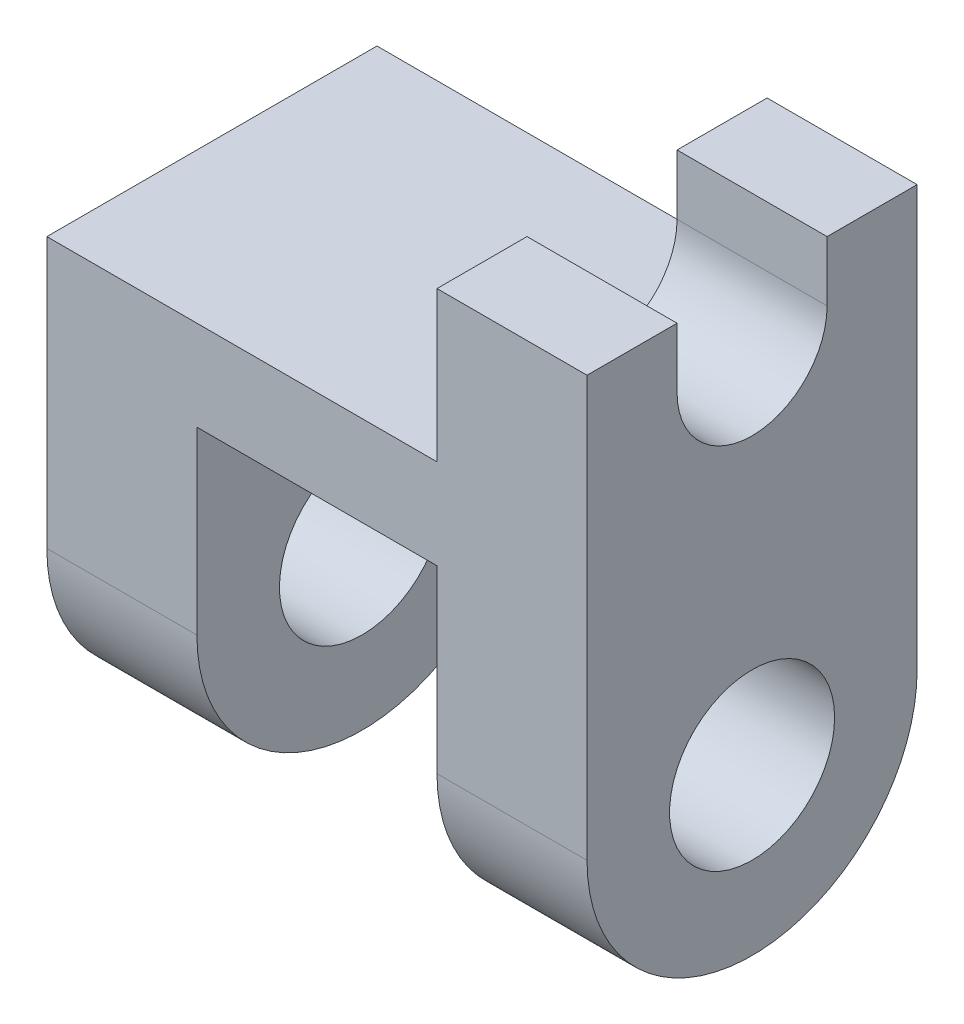
ISO-10303-21;
HEADER;
FILE_DESCRIPTION(('STEP AP214'),'2;1');
FILE_NAME('part.step','',(''),(''),'','','');
FILE_SCHEMA(('AUTOMOTIVE_DESIGN { 1 0 10303 214 1 1 1 1 }'));
ENDSEC;
DATA;
#1=APPLICATION_CONTEXT('core data for automotive mechanical design processes');
#2=APPLICATION_PROTOCOL_DEFINITION('international standard','automotive_design',2000,#1);
#3=PRODUCT_CONTEXT('',#1,'mechanical');
#4=PRODUCT('Part','Part','',(#3));
#5=PRODUCT_RELATED_PRODUCT_CATEGORY('part','',(#4));
#6=PRODUCT_DEFINITION_FORMATION('','',#4);
#7=PRODUCT_DEFINITION_CONTEXT('part definition',#1,'design');
#8=PRODUCT_DEFINITION('design','',#6,#7);
#9=PRODUCT_DEFINITION_SHAPE('','',#8);
#10=(LENGTH_UNIT() NAMED_UNIT(*) SI_UNIT(.MILLI.,.METRE.));
#11=(NAMED_UNIT(*) PLANE_ANGLE_UNIT() SI_UNIT($,.RADIAN.));
#12=(NAMED_UNIT(*) SI_UNIT($,.STERADIAN.) SOLID_ANGLE_UNIT());
#13=UNCERTAINTY_MEASURE_WITH_UNIT(LENGTH_MEASURE(1.E-05),#10,'distance_accuracy_value','');
#14=(GEOMETRIC_REPRESENTATION_CONTEXT(3) GLOBAL_UNCERTAINTY_ASSIGNED_CONTEXT((#13)) GLOBAL_UNIT_ASSIGNED_CONTEXT((#10,
#11,#12)) REPRESENTATION_CONTEXT('',''));
#15=CARTESIAN_POINT('',(0.,0.,0.));
#16=DIRECTION('',(0.,0.,1.));
#17=DIRECTION('',(1.,0.,0.));
#18=AXIS2_PLACEMENT_3D('',#15,#16,#17);
#19=CARTESIAN_POINT('',(36.,32.,22.));
#20=DIRECTION('',(0.,-1.,0.));
#21=DIRECTION('',(0.,0.,-1.));
#22=AXIS2_PLACEMENT_3D('',#19,#20,#21);
#23=PLANE('',#22);
#24=DIRECTION('',(1.,0.,0.));
#25=VECTOR('',#24,1.);
#26=CARTESIAN_POINT('',(-167.635824222232,32.,10.));
#27=LINE('',#26,#25);
#28=CARTESIAN_POINT('',(16.,32.,10.));
#29=VERTEX_POINT('',#28);
#30=CARTESIAN_POINT('',(36.,32.,10.));
#31=VERTEX_POINT('',#30);
#32=EDGE_CURVE('E161',#29,#31,#27,.T.);
#33=ORIENTED_EDGE('',*,*,#32,.F.);
#34=DIRECTION('',(0.,0.,-1.));
#35=VECTOR('',#34,1.);
#36=CARTESIAN_POINT('',(16.,32.,22.));
#37=LINE('',#36,#35);
#38=CARTESIAN_POINT('',(16.,32.,22.));
#39=VERTEX_POINT('',#38);
#40=EDGE_CURVE('E147',#39,#29,#37,.T.);
#41=ORIENTED_EDGE('',*,*,#40,.F.);
#42=DIRECTION('',(-1.,0.,0.));
#43=VECTOR('',#42,1.);
#44=CARTESIAN_POINT('',(36.,32.,22.));
#45=LINE('',#44,#43);
#46=CARTESIAN_POINT('',(36.,32.,22.));
#47=VERTEX_POINT('',#46);
#48=EDGE_CURVE('E224',#47,#39,#45,.T.);
#49=ORIENTED_EDGE('',*,*,#48,.F.);
#50=DIRECTION('',(0.,0.,-1.));
#51=VECTOR('',#50,1.);
#52=CARTESIAN_POINT('',(36.,32.,22.));
#53=LINE('',#52,#51);
#54=EDGE_CURVE('E11',#47,#31,#53,.T.);
#55=ORIENTED_EDGE('',*,*,#54,.T.);
#56=EDGE_LOOP('',(#33,#41,#49,#55));
#57=FACE_BOUND('',#56,.T.);
#58=ADVANCED_FACE('F39',(#57),#23,.F.);
#59=CARTESIAN_POINT('',(16.,32.,22.));
#60=DIRECTION('',(1.,0.,0.));
#61=DIRECTION('',(0.,0.,-1.));
#62=AXIS2_PLACEMENT_3D('',#59,#60,#61);
#63=PLANE('',#62);
#64=ORIENTED_EDGE('',*,*,#40,.T.);
#65=DIRECTION('',(0.,-1.,0.));
#66=VECTOR('',#65,1.);
#67=CARTESIAN_POINT('',(16.,24.,10.));
#68=LINE('',#67,#66);
#69=CARTESIAN_POINT('',(16.,24.,10.));
#70=VERTEX_POINT('',#69);
#71=EDGE_CURVE('E140',#29,#70,#68,.T.);
#72=ORIENTED_EDGE('',*,*,#71,.T.);
#73=CARTESIAN_POINT('',(16.,24.,0.));
#74=DIRECTION('',(1.,0.,0.));
#75=DIRECTION('',(0.,0.,-1.));
#76=AXIS2_PLACEMENT_3D('',#73,#74,#75);
#77=CIRCLE('',#76,10.);
#78=CARTESIAN_POINT('',(16.,24.,-10.));
#79=VERTEX_POINT('',#78);
#80=EDGE_CURVE('E145',#70,#79,#77,.T.);
#81=ORIENTED_EDGE('',*,*,#80,.T.);
#82=DIRECTION('',(0.,1.,0.));
#83=VECTOR('',#82,1.);
#84=CARTESIAN_POINT('',(16.,24.,-10.));
#85=LINE('',#84,#83);
#86=CARTESIAN_POINT('',(16.,32.,-10.));
#87=VERTEX_POINT('',#86);
#88=EDGE_CURVE('E157',#79,#87,#85,.T.);
#89=ORIENTED_EDGE('',*,*,#88,.T.);
#90=CARTESIAN_POINT('',(16.,32.,-22.));
#91=VERTEX_POINT('',#90);
#92=EDGE_CURVE('E252',#87,#91,#37,.T.);
#93=ORIENTED_EDGE('',*,*,#92,.T.);
#94=DIRECTION('',(0.,-1.,0.));
#95=VECTOR('',#94,1.);
#96=CARTESIAN_POINT('',(16.,32.,-22.));
#97=LINE('',#96,#95);
#98=CARTESIAN_POINT('',(16.,12.,-22.));
#99=VERTEX_POINT('',#98);
#100=EDGE_CURVE('E239',#91,#99,#97,.T.);
#101=ORIENTED_EDGE('',*,*,#100,.T.);
#102=DIRECTION('',(0.,0.,-1.));
#103=VECTOR('',#102,1.);
#104=CARTESIAN_POINT('',(16.,12.,22.));
#105=LINE('',#104,#103);
#106=CARTESIAN_POINT('',(16.,12.,22.));
#107=VERTEX_POINT('',#106);
#108=EDGE_CURVE('E248',#107,#99,#105,.T.);
#109=ORIENTED_EDGE('',*,*,#108,.F.);
#110=DIRECTION('',(0.,-1.,0.));
#111=VECTOR('',#110,1.);
#112=CARTESIAN_POINT('',(16.,32.,22.));
#113=LINE('',#112,#111);
#114=EDGE_CURVE('E221',#39,#107,#113,.T.);
#115=ORIENTED_EDGE('',*,*,#114,.F.);
#116=EDGE_LOOP('',(#64,#72,#81,#89,#93,#101,#109,#115));
#117=FACE_BOUND('',#116,.T.);
#118=ADVANCED_FACE('F142',(#117),#63,.F.);
#119=CARTESIAN_POINT('',(-36.,0.,22.));
#120=DIRECTION('',(0.,1.,0.));
#121=DIRECTION('',(0.,0.,1.));
#122=AXIS2_PLACEMENT_3D('',#119,#120,#121);
#123=PLANE('',#122);
#124=DIRECTION('',(0.,0.,1.));
#125=VECTOR('',#124,1.);
#126=CARTESIAN_POINT('',(-16.,0.,22.));
#127=LINE('',#126,#125);
#128=CARTESIAN_POINT('',(-16.,0.,-22.));
#129=VERTEX_POINT('',#128);
#130=CARTESIAN_POINT('',(-16.,0.,22.));
#131=VERTEX_POINT('',#130);
#132=EDGE_CURVE('E193',#129,#131,#127,.T.);
#133=ORIENTED_EDGE('',*,*,#132,.F.);
#134=DIRECTION('',(1.,0.,0.));
#135=VECTOR('',#134,1.);
#136=CARTESIAN_POINT('',(-36.,0.,-22.));
#137=LINE('',#136,#135);
#138=CARTESIAN_POINT('',(16.,0.,-22.));
#139=VERTEX_POINT('',#138);
#140=EDGE_CURVE('E222',#129,#139,#137,.T.);
#141=ORIENTED_EDGE('',*,*,#140,.T.);
#142=DIRECTION('',(0.,0.,-1.));
#143=VECTOR('',#142,1.);
#144=CARTESIAN_POINT('',(16.,0.,22.));
#145=LINE('',#144,#143);
#146=CARTESIAN_POINT('',(16.,0.,22.));
#147=VERTEX_POINT('',#146);
#148=EDGE_CURVE('E203',#147,#139,#145,.T.);
#149=ORIENTED_EDGE('',*,*,#148,.F.);
#150=DIRECTION('',(1.,0.,0.));
#151=VECTOR('',#150,1.);
#152=CARTESIAN_POINT('',(-36.,0.,22.));
#153=LINE('',#152,#151);
#154=EDGE_CURVE('E233',#131,#147,#153,.T.);
#155=ORIENTED_EDGE('',*,*,#154,.F.);
#156=EDGE_LOOP('',(#133,#141,#149,#155));
#157=FACE_BOUND('',#156,.T.);
#158=ADVANCED_FACE('F303',(#157),#123,.F.);
#159=CARTESIAN_POINT('',(36.,0.,22.));
#160=DIRECTION('',(-1.,0.,0.));
#161=DIRECTION('',(0.,0.,1.));
#162=AXIS2_PLACEMENT_3D('',#159,#160,#161);
#163=PLANE('',#162);
#164=DIRECTION('',(0.,1.,0.));
#165=VECTOR('',#164,1.);
#166=CARTESIAN_POINT('',(36.,24.,-10.));
#167=LINE('',#166,#165);
#168=CARTESIAN_POINT('',(36.,24.,-10.));
#169=VERTEX_POINT('',#168);
#170=CARTESIAN_POINT('',(36.,32.,-10.));
#171=VERTEX_POINT('',#170);
#172=EDGE_CURVE('E53',#169,#171,#167,.T.);
#173=ORIENTED_EDGE('',*,*,#172,.F.);
#174=CARTESIAN_POINT('',(36.,24.,0.));
#175=DIRECTION('',(1.,0.,0.));
#176=DIRECTION('',(0.,0.,-1.));
#177=AXIS2_PLACEMENT_3D('',#174,#175,#176);
#178=CIRCLE('',#177,10.);
#179=CARTESIAN_POINT('',(36.,24.,10.));
#180=VERTEX_POINT('',#179);
#181=EDGE_CURVE('E59',#180,#169,#178,.T.);
#182=ORIENTED_EDGE('',*,*,#181,.F.);
#183=DIRECTION('',(0.,-1.,0.));
#184=VECTOR('',#183,1.);
#185=CARTESIAN_POINT('',(36.,24.,10.));
#186=LINE('',#185,#184);
#187=EDGE_CURVE('E163',#31,#180,#186,.T.);
#188=ORIENTED_EDGE('',*,*,#187,.F.);
#189=ORIENTED_EDGE('',*,*,#54,.F.);
#190=DIRECTION('',(0.,1.,0.));
#191=VECTOR('',#190,1.);
#192=CARTESIAN_POINT('',(36.,0.,22.));
#193=LINE('',#192,#191);
#194=CARTESIAN_POINT('',(36.,-24.,22.));
#195=VERTEX_POINT('',#194);
#196=EDGE_CURVE('E218',#195,#47,#193,.T.);
#197=ORIENTED_EDGE('',*,*,#196,.F.);
#198=CARTESIAN_POINT('',(36.,-24.,0.));
#199=DIRECTION('',(1.,0.,0.));
#200=DIRECTION('',(0.,0.,-1.));
#201=AXIS2_PLACEMENT_3D('',#198,#199,#200);
#202=CIRCLE('',#201,22.);
#203=CARTESIAN_POINT('',(36.,-24.,-22.));
#204=VERTEX_POINT('',#203);
#205=EDGE_CURVE('E175',#195,#204,#202,.T.);
#206=ORIENTED_EDGE('',*,*,#205,.T.);
#207=DIRECTION('',(0.,1.,0.));
#208=VECTOR('',#207,1.);
#209=CARTESIAN_POINT('',(36.,0.,-22.));
#210=LINE('',#209,#208);
#211=CARTESIAN_POINT('',(36.,32.,-22.));
#212=VERTEX_POINT('',#211);
#213=EDGE_CURVE('E210',#204,#212,#210,.T.);
#214=ORIENTED_EDGE('',*,*,#213,.T.);
#215=EDGE_CURVE('E50',#171,#212,#53,.T.);
#216=ORIENTED_EDGE('',*,*,#215,.F.);
#217=EDGE_LOOP('',(#173,#182,#188,#189,#197,#206,#214,#216));
#218=FACE_BOUND('',#217,.T.);
#219=CARTESIAN_POINT('',(36.,-24.,0.));
#220=DIRECTION('',(1.,0.,0.));
#221=DIRECTION('',(0.,0.,-1.));
#222=AXIS2_PLACEMENT_3D('',#219,#220,#221);
#223=CIRCLE('',#222,11.);
#224=CARTESIAN_POINT('',(36.,-24.,-11.));
#225=VERTEX_POINT('',#224);
#226=EDGE_CURVE('E162',#225,#225,#223,.T.);
#227=ORIENTED_EDGE('',*,*,#226,.F.);
#228=EDGE_LOOP('',(#227));
#229=FACE_BOUND('',#228,.T.);
#230=ADVANCED_FACE('F41',(#218,#229),#163,.F.);
#231=ORIENTED_EDGE('',*,*,#92,.F.);
#232=DIRECTION('',(1.,0.,0.));
#233=VECTOR('',#232,1.);
#234=CARTESIAN_POINT('',(-167.635824222232,32.,-10.));
#235=LINE('',#234,#233);
#236=EDGE_CURVE('E354',#87,#171,#235,.T.);
#237=ORIENTED_EDGE('',*,*,#236,.T.);
#238=ORIENTED_EDGE('',*,*,#215,.T.);
#239=DIRECTION('',(-1.,0.,0.));
#240=VECTOR('',#239,1.);
#241=CARTESIAN_POINT('',(36.,32.,-22.));
#242=LINE('',#241,#240);
#243=EDGE_CURVE('E240',#212,#91,#242,.T.);
#244=ORIENTED_EDGE('',*,*,#243,.T.);
#245=EDGE_LOOP('',(#231,#237,#238,#244));
#246=FACE_BOUND('',#245,.T.);
#247=ADVANCED_FACE('F259',(#246),#23,.F.);
#248=CARTESIAN_POINT('',(16.,12.,22.));
#249=DIRECTION('',(0.,-1.,0.));
#250=DIRECTION('',(1.,0.,0.));
#251=AXIS2_PLACEMENT_3D('',#248,#249,#250);
#252=PLANE('',#251);
#253=DIRECTION('',(-1.,0.,0.));
#254=VECTOR('',#253,1.);
#255=CARTESIAN_POINT('',(16.,12.,-22.));
#256=LINE('',#255,#254);
#257=CARTESIAN_POINT('',(-36.,12.,-22.));
#258=VERTEX_POINT('',#257);
#259=EDGE_CURVE('E245',#99,#258,#256,.T.);
#260=ORIENTED_EDGE('',*,*,#259,.T.);
#261=DIRECTION('',(0.,0.,-1.));
#262=VECTOR('',#261,1.);
#263=CARTESIAN_POINT('',(-36.,12.,22.));
#264=LINE('',#263,#262);
#265=CARTESIAN_POINT('',(-36.,12.,22.));
#266=VERTEX_POINT('',#265);
#267=EDGE_CURVE('E234',#266,#258,#264,.T.);
#268=ORIENTED_EDGE('',*,*,#267,.F.);
#269=DIRECTION('',(-1.,0.,0.));
#270=VECTOR('',#269,1.);
#271=CARTESIAN_POINT('',(16.,12.,22.));
#272=LINE('',#271,#270);
#273=EDGE_CURVE('E227',#107,#266,#272,.T.);
#274=ORIENTED_EDGE('',*,*,#273,.F.);
#275=ORIENTED_EDGE('',*,*,#108,.T.);
#276=EDGE_LOOP('',(#260,#268,#274,#275));
#277=FACE_BOUND('',#276,.T.);
#278=ADVANCED_FACE('F269',(#277),#252,.F.);
#279=CARTESIAN_POINT('',(-36.,12.,22.));
#280=DIRECTION('',(1.,0.,0.));
#281=DIRECTION('',(0.,1.,0.));
#282=AXIS2_PLACEMENT_3D('',#279,#280,#281);
#283=PLANE('',#282);
#284=DIRECTION('',(0.,-1.,0.));
#285=VECTOR('',#284,1.);
#286=CARTESIAN_POINT('',(-36.,12.,-22.));
#287=LINE('',#286,#285);
#288=CARTESIAN_POINT('',(-36.,-24.,-22.));
#289=VERTEX_POINT('',#288);
#290=EDGE_CURVE('E242',#258,#289,#287,.T.);
#291=ORIENTED_EDGE('',*,*,#290,.T.);
#292=CARTESIAN_POINT('',(-36.,-24.,0.));
#293=DIRECTION('',(-1.,0.,0.));
#294=DIRECTION('',(0.,-1.,0.));
#295=AXIS2_PLACEMENT_3D('',#292,#293,#294);
#296=CIRCLE('',#295,22.);
#297=CARTESIAN_POINT('',(-36.,-24.,22.));
#298=VERTEX_POINT('',#297);
#299=EDGE_CURVE('E185',#289,#298,#296,.T.);
#300=ORIENTED_EDGE('',*,*,#299,.T.);
#301=DIRECTION('',(0.,-1.,0.));
#302=VECTOR('',#301,1.);
#303=CARTESIAN_POINT('',(-36.,12.,22.));
#304=LINE('',#303,#302);
#305=EDGE_CURVE('E230',#266,#298,#304,.T.);
#306=ORIENTED_EDGE('',*,*,#305,.F.);
#307=ORIENTED_EDGE('',*,*,#267,.T.);
#308=EDGE_LOOP('',(#291,#300,#306,#307));
#309=FACE_BOUND('',#308,.T.);
#310=CARTESIAN_POINT('',(-36.,-24.,0.));
#311=DIRECTION('',(-1.,0.,0.));
#312=DIRECTION('',(0.,-1.,0.));
#313=AXIS2_PLACEMENT_3D('',#310,#311,#312);
#314=CIRCLE('',#313,11.);
#315=CARTESIAN_POINT('',(-36.,-35.,0.));
#316=VERTEX_POINT('',#315);
#317=EDGE_CURVE('E176',#316,#316,#314,.T.);
#318=ORIENTED_EDGE('',*,*,#317,.F.);
#319=EDGE_LOOP('',(#318));
#320=FACE_BOUND('',#319,.T.);
#321=ADVANCED_FACE('F272',(#309,#320),#283,.F.);
#322=CARTESIAN_POINT('',(0.,0.,22.));
#323=DIRECTION('',(0.,0.,1.));
#324=DIRECTION('',(1.,0.,0.));
#325=AXIS2_PLACEMENT_3D('',#322,#323,#324);
#326=PLANE('',#325);
#327=ORIENTED_EDGE('',*,*,#196,.T.);
#328=ORIENTED_EDGE('',*,*,#48,.T.);
#329=ORIENTED_EDGE('',*,*,#114,.T.);
#330=ORIENTED_EDGE('',*,*,#273,.T.);
#331=ORIENTED_EDGE('',*,*,#305,.T.);
#332=DIRECTION('',(-1.,0.,0.));
#333=VECTOR('',#332,1.);
#334=CARTESIAN_POINT('',(-36.,-24.,22.));
#335=LINE('',#334,#333);
#336=CARTESIAN_POINT('',(-16.,-24.,22.));
#337=VERTEX_POINT('',#336);
#338=EDGE_CURVE('E191',#337,#298,#335,.T.);
#339=ORIENTED_EDGE('',*,*,#338,.F.);
#340=DIRECTION('',(0.,1.,0.));
#341=VECTOR('',#340,1.);
#342=CARTESIAN_POINT('',(-16.,-24.,22.));
#343=LINE('',#342,#341);
#344=EDGE_CURVE('E197',#337,#131,#343,.T.);
#345=ORIENTED_EDGE('',*,*,#344,.T.);
#346=ORIENTED_EDGE('',*,*,#154,.T.);
#347=DIRECTION('',(0.,1.,0.));
#348=VECTOR('',#347,1.);
#349=CARTESIAN_POINT('',(16.,-24.,22.));
#350=LINE('',#349,#348);
#351=CARTESIAN_POINT('',(16.,-24.,22.));
#352=VERTEX_POINT('',#351);
#353=EDGE_CURVE('E189',#352,#147,#350,.T.);
#354=ORIENTED_EDGE('',*,*,#353,.F.);
#355=DIRECTION('',(-1.,0.,0.));
#356=VECTOR('',#355,1.);
#357=CARTESIAN_POINT('',(36.,-24.,22.));
#358=LINE('',#357,#356);
#359=EDGE_CURVE('E216',#195,#352,#358,.T.);
#360=ORIENTED_EDGE('',*,*,#359,.F.);
#361=EDGE_LOOP('',(#327,#328,#329,#330,#331,#339,#345,#346,#354,#360));
#362=FACE_BOUND('',#361,.T.);
#363=ADVANCED_FACE('F277',(#362),#326,.T.);
#364=CARTESIAN_POINT('',(0.,0.,-22.));
#365=DIRECTION('',(0.,0.,1.));
#366=DIRECTION('',(1.,0.,0.));
#367=AXIS2_PLACEMENT_3D('',#364,#365,#366);
#368=PLANE('',#367);
#369=ORIENTED_EDGE('',*,*,#213,.F.);
#370=DIRECTION('',(1.,0.,0.));
#371=VECTOR('',#370,1.);
#372=CARTESIAN_POINT('',(16.,-24.,-22.));
#373=LINE('',#372,#371);
#374=CARTESIAN_POINT('',(16.,-24.,-22.));
#375=VERTEX_POINT('',#374);
#376=EDGE_CURVE('E214',#375,#204,#373,.T.);
#377=ORIENTED_EDGE('',*,*,#376,.F.);
#378=DIRECTION('',(0.,1.,0.));
#379=VECTOR('',#378,1.);
#380=CARTESIAN_POINT('',(16.,-24.,-22.));
#381=LINE('',#380,#379);
#382=EDGE_CURVE('E208',#375,#139,#381,.T.);
#383=ORIENTED_EDGE('',*,*,#382,.T.);
#384=ORIENTED_EDGE('',*,*,#140,.F.);
#385=DIRECTION('',(0.,1.,0.));
#386=VECTOR('',#385,1.);
#387=CARTESIAN_POINT('',(-16.,-24.,-22.));
#388=LINE('',#387,#386);
#389=CARTESIAN_POINT('',(-16.,-24.,-22.));
#390=VERTEX_POINT('',#389);
#391=EDGE_CURVE('E205',#390,#129,#388,.T.);
#392=ORIENTED_EDGE('',*,*,#391,.F.);
#393=DIRECTION('',(1.,0.,0.));
#394=VECTOR('',#393,1.);
#395=CARTESIAN_POINT('',(-16.,-24.,-22.));
#396=LINE('',#395,#394);
#397=EDGE_CURVE('E192',#289,#390,#396,.T.);
#398=ORIENTED_EDGE('',*,*,#397,.F.);
#399=ORIENTED_EDGE('',*,*,#290,.F.);
#400=ORIENTED_EDGE('',*,*,#259,.F.);
#401=ORIENTED_EDGE('',*,*,#100,.F.);
#402=ORIENTED_EDGE('',*,*,#243,.F.);
#403=EDGE_LOOP('',(#369,#377,#383,#384,#392,#398,#399,#400,#401,#402));
#404=FACE_BOUND('',#403,.T.);
#405=ADVANCED_FACE('F265',(#404),#368,.F.);
#406=CARTESIAN_POINT('',(16.,-24.,22.));
#407=DIRECTION('',(1.,0.,0.));
#408=DIRECTION('',(0.,0.,-1.));
#409=AXIS2_PLACEMENT_3D('',#406,#407,#408);
#410=PLANE('',#409);
#411=ORIENTED_EDGE('',*,*,#382,.F.);
#412=CARTESIAN_POINT('',(16.,-24.,0.));
#413=DIRECTION('',(1.,0.,0.));
#414=DIRECTION('',(0.,0.,-1.));
#415=AXIS2_PLACEMENT_3D('',#412,#413,#414);
#416=CIRCLE('',#415,22.);
#417=EDGE_CURVE('E172',#352,#375,#416,.T.);
#418=ORIENTED_EDGE('',*,*,#417,.F.);
#419=ORIENTED_EDGE('',*,*,#353,.T.);
#420=ORIENTED_EDGE('',*,*,#148,.T.);
#421=EDGE_LOOP('',(#411,#418,#419,#420));
#422=FACE_BOUND('',#421,.T.);
#423=CARTESIAN_POINT('',(16.,-24.,0.));
#424=DIRECTION('',(1.,0.,0.));
#425=DIRECTION('',(0.,0.,-1.));
#426=AXIS2_PLACEMENT_3D('',#423,#424,#425);
#427=CIRCLE('',#426,11.);
#428=CARTESIAN_POINT('',(16.,-24.,-11.));
#429=VERTEX_POINT('',#428);
#430=EDGE_CURVE('E168',#429,#429,#427,.T.);
#431=ORIENTED_EDGE('',*,*,#430,.T.);
#432=EDGE_LOOP('',(#431));
#433=FACE_BOUND('',#432,.T.);
#434=ADVANCED_FACE('F290',(#422,#433),#410,.F.);
#435=CARTESIAN_POINT('',(-16.,-24.,22.));
#436=DIRECTION('',(-1.,0.,0.));
#437=DIRECTION('',(0.,0.,1.));
#438=AXIS2_PLACEMENT_3D('',#435,#436,#437);
#439=PLANE('',#438);
#440=ORIENTED_EDGE('',*,*,#344,.F.);
#441=CARTESIAN_POINT('',(-16.,-24.,0.));
#442=DIRECTION('',(-1.,0.,0.));
#443=DIRECTION('',(0.,-1.,0.));
#444=AXIS2_PLACEMENT_3D('',#441,#442,#443);
#445=CIRCLE('',#444,22.);
#446=EDGE_CURVE('E184',#390,#337,#445,.T.);
#447=ORIENTED_EDGE('',*,*,#446,.F.);
#448=ORIENTED_EDGE('',*,*,#391,.T.);
#449=ORIENTED_EDGE('',*,*,#132,.T.);
#450=EDGE_LOOP('',(#440,#447,#448,#449));
#451=FACE_BOUND('',#450,.T.);
#452=CARTESIAN_POINT('',(-16.,-24.,0.));
#453=DIRECTION('',(-1.,0.,0.));
#454=DIRECTION('',(0.,-1.,0.));
#455=AXIS2_PLACEMENT_3D('',#452,#453,#454);
#456=CIRCLE('',#455,11.);
#457=CARTESIAN_POINT('',(-16.,-35.,0.));
#458=VERTEX_POINT('',#457);
#459=EDGE_CURVE('E177',#458,#458,#456,.T.);
#460=ORIENTED_EDGE('',*,*,#459,.T.);
#461=EDGE_LOOP('',(#460));
#462=FACE_BOUND('',#461,.T.);
#463=ADVANCED_FACE('F281',(#451,#462),#439,.F.);
#464=CARTESIAN_POINT('',(-16.,-24.,0.));
#465=DIRECTION('',(-1.,0.,0.));
#466=DIRECTION('',(0.,-1.,0.));
#467=AXIS2_PLACEMENT_3D('',#464,#465,#466);
#468=CYLINDRICAL_SURFACE('',#467,22.);
#469=ORIENTED_EDGE('',*,*,#397,.T.);
#470=ORIENTED_EDGE('',*,*,#446,.T.);
#471=ORIENTED_EDGE('',*,*,#338,.T.);
#472=ORIENTED_EDGE('',*,*,#299,.F.);
#473=EDGE_LOOP('',(#469,#470,#471,#472));
#474=FACE_BOUND('',#473,.T.);
#475=ADVANCED_FACE('F279',(#474),#468,.T.);
#476=CARTESIAN_POINT('',(-16.,-24.,0.));
#477=DIRECTION('',(-1.,0.,0.));
#478=DIRECTION('',(0.,-1.,0.));
#479=AXIS2_PLACEMENT_3D('',#476,#477,#478);
#480=CYLINDRICAL_SURFACE('',#479,11.);
#481=ORIENTED_EDGE('',*,*,#317,.T.);
#482=EDGE_LOOP('',(#481));
#483=FACE_BOUND('',#482,.T.);
#484=ORIENTED_EDGE('',*,*,#459,.F.);
#485=EDGE_LOOP('',(#484));
#486=FACE_BOUND('',#485,.T.);
#487=ADVANCED_FACE('F337',(#483,#486),#480,.F.);
#488=CARTESIAN_POINT('',(16.,-24.,0.));
#489=DIRECTION('',(1.,0.,0.));
#490=DIRECTION('',(0.,0.,-1.));
#491=AXIS2_PLACEMENT_3D('',#488,#489,#490);
#492=CYLINDRICAL_SURFACE('',#491,22.);
#493=ORIENTED_EDGE('',*,*,#417,.T.);
#494=ORIENTED_EDGE('',*,*,#376,.T.);
#495=ORIENTED_EDGE('',*,*,#205,.F.);
#496=ORIENTED_EDGE('',*,*,#359,.T.);
#497=EDGE_LOOP('',(#493,#494,#495,#496));
#498=FACE_BOUND('',#497,.T.);
#499=ADVANCED_FACE('F291',(#498),#492,.T.);
#500=CARTESIAN_POINT('',(16.,-24.,0.));
#501=DIRECTION('',(1.,0.,0.));
#502=DIRECTION('',(0.,0.,-1.));
#503=AXIS2_PLACEMENT_3D('',#500,#501,#502);
#504=CYLINDRICAL_SURFACE('',#503,11.);
#505=ORIENTED_EDGE('',*,*,#226,.T.);
#506=EDGE_LOOP('',(#505));
#507=FACE_BOUND('',#506,.T.);
#508=ORIENTED_EDGE('',*,*,#430,.F.);
#509=EDGE_LOOP('',(#508));
#510=FACE_BOUND('',#509,.T.);
#511=ADVANCED_FACE('F342',(#507,#510),#504,.F.);
#512=CARTESIAN_POINT('',(-167.635824222232,24.,10.));
#513=DIRECTION('',(0.,0.,-1.));
#514=DIRECTION('',(-1.,0.,0.));
#515=AXIS2_PLACEMENT_3D('',#512,#513,#514);
#516=PLANE('',#515);
#517=ORIENTED_EDGE('',*,*,#71,.F.);
#518=ORIENTED_EDGE('',*,*,#32,.T.);
#519=ORIENTED_EDGE('',*,*,#187,.T.);
#520=DIRECTION('',(1.,0.,0.));
#521=VECTOR('',#520,1.);
#522=CARTESIAN_POINT('',(-167.635824222232,24.,10.));
#523=LINE('',#522,#521);
#524=EDGE_CURVE('E154',#70,#180,#523,.T.);
#525=ORIENTED_EDGE('',*,*,#524,.F.);
#526=EDGE_LOOP('',(#517,#518,#519,#525));
#527=FACE_BOUND('',#526,.T.);
#528=ADVANCED_FACE('F156',(#527),#516,.T.);
#529=CARTESIAN_POINT('',(-167.635824222232,24.,0.));
#530=DIRECTION('',(1.,0.,0.));
#531=DIRECTION('',(0.,0.,-1.));
#532=AXIS2_PLACEMENT_3D('',#529,#530,#531);
#533=CYLINDRICAL_SURFACE('',#532,10.);
#534=ORIENTED_EDGE('',*,*,#80,.F.);
#535=ORIENTED_EDGE('',*,*,#524,.T.);
#536=ORIENTED_EDGE('',*,*,#181,.T.);
#537=DIRECTION('',(1.,0.,0.));
#538=VECTOR('',#537,1.);
#539=CARTESIAN_POINT('',(-167.635824222232,24.,-10.));
#540=LINE('',#539,#538);
#541=EDGE_CURVE('E159',#79,#169,#540,.T.);
#542=ORIENTED_EDGE('',*,*,#541,.F.);
#543=EDGE_LOOP('',(#534,#535,#536,#542));
#544=FACE_BOUND('',#543,.T.);
#545=ADVANCED_FACE('F153',(#544),#533,.F.);
#546=CARTESIAN_POINT('',(-167.635824222232,24.,-10.));
#547=DIRECTION('',(0.,0.,1.));
#548=DIRECTION('',(1.,0.,0.));
#549=AXIS2_PLACEMENT_3D('',#546,#547,#548);
#550=PLANE('',#549);
#551=ORIENTED_EDGE('',*,*,#88,.F.);
#552=ORIENTED_EDGE('',*,*,#541,.T.);
#553=ORIENTED_EDGE('',*,*,#172,.T.);
#554=ORIENTED_EDGE('',*,*,#236,.F.);
#555=EDGE_LOOP('',(#551,#552,#553,#554));
#556=FACE_BOUND('',#555,.T.);
#557=ADVANCED_FACE('F350',(#556),#550,.T.);
#558=CLOSED_SHELL('',(#58,#118,#158,#230,#247,#278,#321,#363,#405,#434,#463,#475,#487,#499,#511,
#528,#545,#557));
#559=MANIFOLD_SOLID_BREP('B2',#558);
#560=ADVANCED_BREP_SHAPE_REPRESENTATION('',(#18,#559),#14);
#561=SHAPE_DEFINITION_REPRESENTATION(#9,#560);
ENDSEC;
END-ISO-10303-21;
